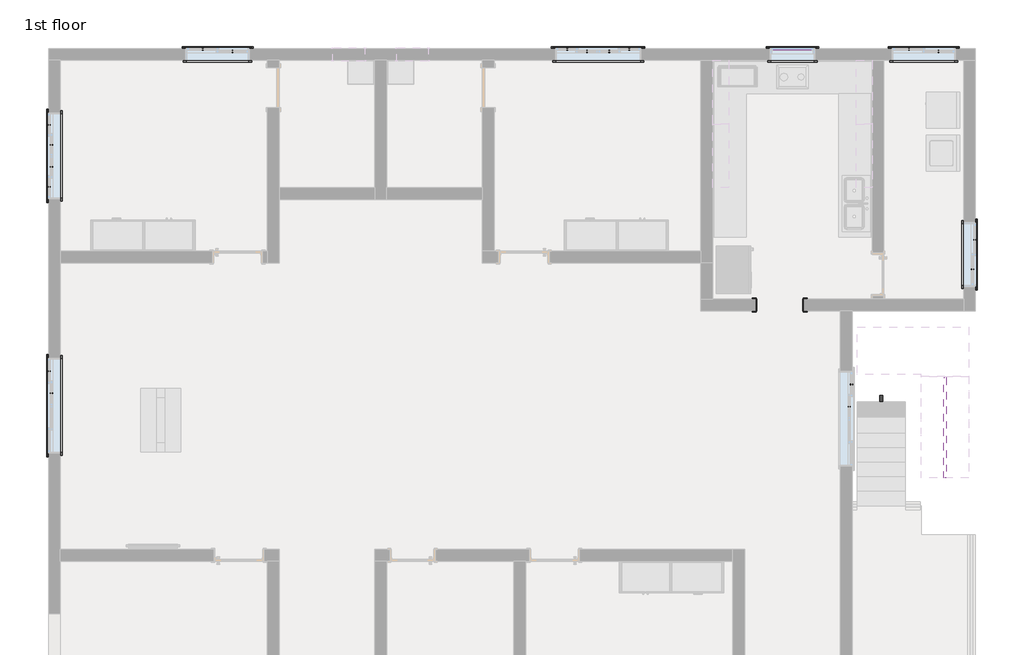
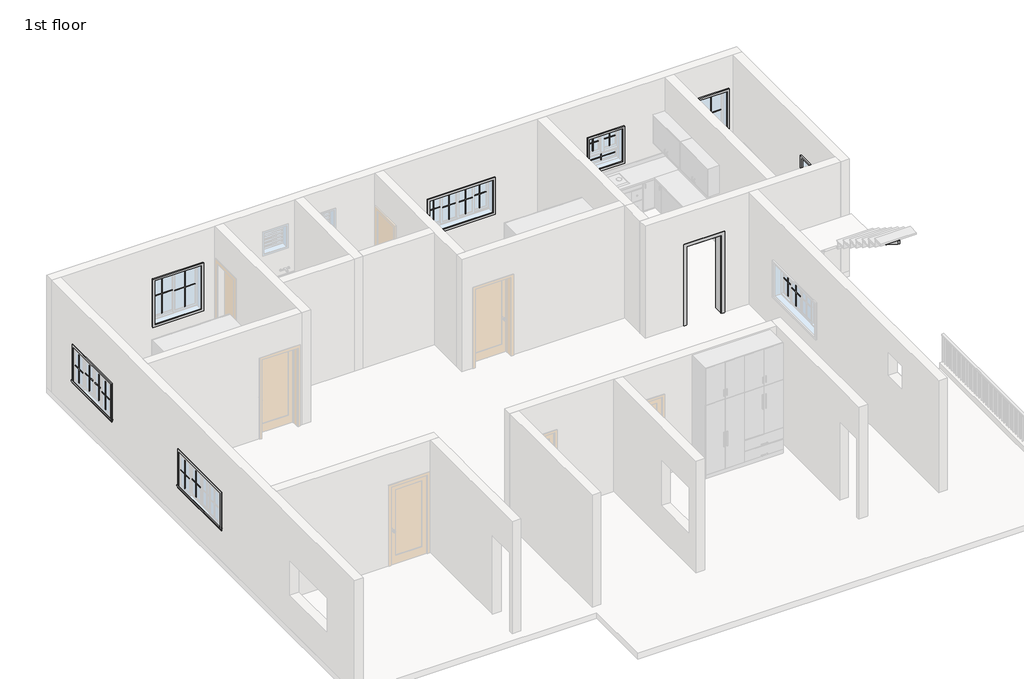
# One storey, part 4 of 4: 36 proxies, 2 members.
"""IFC4 building model written with IfcOpenShell, lengths in millimetres."""

from ifc_helpers import new_model, si_unit, frame, origin, place, context, project, spatial, polyline, outline, extrude, transform, mapped, element, save
from components import muntin_pattern_2x2_muntin_pattern_2x2_6186d23a, muntin_pattern_2x2_muntin_pattern_2x2_31a16349, muntin_pattern_2x2_muntin_pattern_2x2_cf37b409, muntin_pattern_2x2_muntin_pattern_2x2_78ce0566, muntin_pattern_2x2_muntin_pattern_2x2_27bf4e5b, muntin_pattern_2x2_muntin_pattern_2x2_8320156c, proxy_e9bf662a, trim_window_exterior_flat_with_sill_c3f87112, trim_window_exterior_flat_with_sill_3c945769, trim_window_exterior_flat_with_sill_7cfdd449, trim_window_exterior_flat_with_sill_41619996, trim_window_interior_flat_picture_frame_1c33fa8a, trim_window_interior_flat_picture_frame_0edfbaa2, trim_window_interior_flat_picture_frame_f1e0b15b, trim_window_interior_flat_picture_frame_51c85655

model = new_model("IFC4")

# Units and contexts
model_context = context("Model", 3, world=origin())
ifc_project = project(units=[si_unit("LENGTHUNIT", "METRE", prefix="MILLI")], contexts=[model_context])

# Site, building, storey
site = spatial("IfcSite", under=ifc_project)
building = spatial("IfcBuilding", under=site)
storey = spatial("IfcBuildingStorey", under=building, Name="1st floor", Elevation=3810.0)

# Proxies
placement = place(None, origin())
muntin_pattern_2x2_muntin_pattern_2x2_shape = muntin_pattern_2x2_muntin_pattern_2x2_6186d23a(model_context)
element("IfcBuildingElementProxy", 1, Name="Muntin Pattern_2x2 : Muntin Pattern_2x2", ObjectType="Muntin Pattern_2x2 : Muntin Pattern_2x2", at=placement, inside=storey, context=model_context, shape_type="MappedRepresentation", body=[
    mapped(muntin_pattern_2x2_muntin_pattern_2x2_shape, transform((1905.0010838, 7064.4410813, 4806.95), x_axis=(1.0, 0.0, 0.0), y_axis=(0.0, 1.0, 0.0), z_axis=(0.0, 0.0, 1.0))),
])
element("IfcBuildingElementProxy", 2, Name="Muntin Pattern_2x2 : Muntin Pattern_2x2", ObjectType="Muntin Pattern_2x2 : Muntin Pattern_2x2", at=placement, inside=storey, context=model_context, shape_type="MappedRepresentation", body=[
    mapped(muntin_pattern_2x2_muntin_pattern_2x2_shape, transform((2286.0010838, 7019.9910813, 4806.95), x_axis=(1.0, 0.0, 0.0), y_axis=(0.0, 1.0, 0.0), z_axis=(0.0, 0.0, 1.0))),
])
element("IfcBuildingElementProxy", 3, Name="Muntin Pattern_2x2 : Muntin Pattern_2x2", ObjectType="Muntin Pattern_2x2 : Muntin Pattern_2x2", at=placement, inside=storey, context=model_context, shape_type="MappedRepresentation", body=[
    mapped(muntin_pattern_2x2_muntin_pattern_2x2_shape, transform((2711.4510838, 7019.9910813, 4806.95), x_axis=(1.0, 0.0, 0.0), y_axis=(0.0, 1.0, 0.0), z_axis=(0.0, 0.0, 1.0))),
])
element("IfcBuildingElementProxy", 4, Name="Muntin Pattern_2x2 : Muntin Pattern_2x2", ObjectType="Muntin Pattern_2x2 : Muntin Pattern_2x2", at=placement, inside=storey, context=model_context, shape_type="MappedRepresentation", body=[
    mapped(muntin_pattern_2x2_muntin_pattern_2x2_shape, transform((3092.4510838, 7064.4410813, 4806.95), x_axis=(1.0, 0.0, 0.0), y_axis=(0.0, 1.0, 0.0), z_axis=(0.0, 0.0, 1.0))),
])
element("IfcBuildingElementProxy", 5, Name="Muntin Pattern_2x2 : Muntin Pattern_2x2", ObjectType="Muntin Pattern_2x2 : Muntin Pattern_2x2", at=placement, inside=storey, context=model_context, shape_type="MappedRepresentation", body=[
    mapped(muntin_pattern_2x2_muntin_pattern_2x2_shape, transform((-8020.0489162, 4422.8410813, 4806.95), x_axis=(0.0, 1.0, 0.0), y_axis=(-1.0, 0.0, 0.0), z_axis=(0.0, 0.0, 1.0))),
])
element("IfcBuildingElementProxy", 6, Name="Muntin Pattern_2x2 : Muntin Pattern_2x2", ObjectType="Muntin Pattern_2x2 : Muntin Pattern_2x2", at=placement, inside=storey, context=model_context, shape_type="MappedRepresentation", body=[
    mapped(muntin_pattern_2x2_muntin_pattern_2x2_shape, transform((-7975.5989162, 4803.8410813, 4806.95), x_axis=(0.0, 1.0, 0.0), y_axis=(-1.0, 0.0, 0.0), z_axis=(0.0, 0.0, 1.0))),
])
element("IfcBuildingElementProxy", 7, Name="Muntin Pattern_2x2 : Muntin Pattern_2x2", ObjectType="Muntin Pattern_2x2 : Muntin Pattern_2x2", at=placement, inside=storey, context=model_context, shape_type="MappedRepresentation", body=[
    mapped(muntin_pattern_2x2_muntin_pattern_2x2_shape, transform((-7975.5989162, 5229.2910813, 4806.95), x_axis=(0.0, 1.0, 0.0), y_axis=(-1.0, 0.0, 0.0), z_axis=(0.0, 0.0, 1.0))),
])
element("IfcBuildingElementProxy", 8, Name="Muntin Pattern_2x2 : Muntin Pattern_2x2", ObjectType="Muntin Pattern_2x2 : Muntin Pattern_2x2", at=placement, inside=storey, context=model_context, shape_type="MappedRepresentation", body=[
    mapped(muntin_pattern_2x2_muntin_pattern_2x2_shape, transform((-8020.0489162, 5610.2910813, 4806.95), x_axis=(0.0, 1.0, 0.0), y_axis=(-1.0, 0.0, 0.0), z_axis=(0.0, 0.0, 1.0))),
])
muntin_pattern_2x2_muntin_pattern_2x2_2_shape = muntin_pattern_2x2_muntin_pattern_2x2_31a16349(model_context)
element("IfcBuildingElementProxy", 9, Name="Muntin Pattern_2x2 : Muntin Pattern_2x2", ObjectType="Muntin Pattern_2x2 : Muntin Pattern_2x2", at=placement, inside=storey, context=model_context, shape_type="MappedRepresentation", body=[
    mapped(muntin_pattern_2x2_muntin_pattern_2x2_2_shape, transform((-7975.5989162, 463.6160813, 4806.95), x_axis=(0.0, 1.0, 0.0), y_axis=(-1.0, 0.0, 0.0), z_axis=(0.0, 0.0, 1.0))),
])
element("IfcBuildingElementProxy", 10, Name="Muntin Pattern_2x2 : Muntin Pattern_2x2", ObjectType="Muntin Pattern_2x2 : Muntin Pattern_2x2", at=placement, inside=storey, context=model_context, shape_type="MappedRepresentation", body=[
    mapped(muntin_pattern_2x2_muntin_pattern_2x2_2_shape, transform((-8020.0489162, 889.0660813, 4806.95), x_axis=(0.0, 1.0, 0.0), y_axis=(-1.0, 0.0, 0.0), z_axis=(0.0, 0.0, 1.0))),
])
element("IfcBuildingElementProxy", 11, Name="Muntin Pattern_2x2 : Muntin Pattern_2x2", ObjectType="Muntin Pattern_2x2 : Muntin Pattern_2x2", at=placement, inside=storey, context=model_context, shape_type="MappedRepresentation", body=[
    mapped(muntin_pattern_2x2_muntin_pattern_2x2_2_shape, transform((7353.3010838, 635.0660813, 4806.95), x_axis=(0.0, -1.0, 0.0), y_axis=(1.0, 0.0, 0.0), z_axis=(0.0, 0.0, 1.0))),
])
element("IfcBuildingElementProxy", 12, Name="Muntin Pattern_2x2 : Muntin Pattern_2x2", ObjectType="Muntin Pattern_2x2 : Muntin Pattern_2x2", at=placement, inside=storey, context=model_context, shape_type="MappedRepresentation", body=[
    mapped(muntin_pattern_2x2_muntin_pattern_2x2_2_shape, transform((7308.8510838, 209.6160813, 4806.95), x_axis=(0.0, -1.0, 0.0), y_axis=(1.0, 0.0, 0.0), z_axis=(0.0, 0.0, 1.0))),
])
muntin_pattern_2x2_muntin_pattern_2x2_3_shape = muntin_pattern_2x2_muntin_pattern_2x2_cf37b409(model_context)
element("IfcBuildingElementProxy", 13, Name="Muntin Pattern_2x2 : Muntin Pattern_2x2", ObjectType="Muntin Pattern_2x2 : Muntin Pattern_2x2", at=placement, inside=storey, context=model_context, shape_type="MappedRepresentation", body=[
    mapped(muntin_pattern_2x2_muntin_pattern_2x2_3_shape, transform((9018.5885838, 7019.9910813, 4806.95), x_axis=(1.0, 0.0, 0.0), y_axis=(0.0, 1.0, 0.0), z_axis=(0.0, 0.0, 1.0))),
])
element("IfcBuildingElementProxy", 14, Name="Muntin Pattern_2x2 : Muntin Pattern_2x2", ObjectType="Muntin Pattern_2x2 : Muntin Pattern_2x2", at=placement, inside=storey, context=model_context, shape_type="MappedRepresentation", body=[
    mapped(muntin_pattern_2x2_muntin_pattern_2x2_3_shape, transform((8450.2635838, 7064.4410813, 4806.95), x_axis=(1.0, 0.0, 0.0), y_axis=(0.0, 1.0, 0.0), z_axis=(0.0, 0.0, 1.0))),
])
element("IfcBuildingElementProxy", 15, Name="Muntin Pattern_2x2 : Muntin Pattern_2x2", ObjectType="Muntin Pattern_2x2 : Muntin Pattern_2x2", at=placement, inside=storey, context=model_context, shape_type="MappedRepresentation", body=[
    mapped(muntin_pattern_2x2_muntin_pattern_2x2_3_shape, transform((9671.0510838, 2840.1035813, 4806.95), x_axis=(0.0, -1.0, 0.0), y_axis=(1.0, 0.0, 0.0), z_axis=(0.0, 0.0, 1.0))),
])
element("IfcBuildingElementProxy", 16, Name="Muntin Pattern_2x2 : Muntin Pattern_2x2", ObjectType="Muntin Pattern_2x2 : Muntin Pattern_2x2", at=placement, inside=storey, context=model_context, shape_type="MappedRepresentation", body=[
    mapped(muntin_pattern_2x2_muntin_pattern_2x2_3_shape, transform((9715.5010838, 3408.4285813, 4806.95), x_axis=(0.0, -1.0, 0.0), y_axis=(1.0, 0.0, 0.0), z_axis=(0.0, 0.0, 1.0))),
])
element("IfcBuildingElementProxy", 17, Name="Muntin Pattern_2x2 : Muntin Pattern_2x2", ObjectType="Muntin Pattern_2x2 : Muntin Pattern_2x2", at=placement, inside=storey, context=model_context, shape_type="MappedRepresentation", body=[
    mapped(muntin_pattern_2x2_muntin_pattern_2x2_3_shape, transform((-4506.9114162, 7019.9910813, 4806.95), x_axis=(1.0, 0.0, 0.0), y_axis=(0.0, 1.0, 0.0), z_axis=(0.0, 0.0, 1.0))),
])
element("IfcBuildingElementProxy", 18, Name="Muntin Pattern_2x2 : Muntin Pattern_2x2", ObjectType="Muntin Pattern_2x2 : Muntin Pattern_2x2", at=placement, inside=storey, context=model_context, shape_type="MappedRepresentation", body=[
    mapped(muntin_pattern_2x2_muntin_pattern_2x2_3_shape, transform((-5075.2364162, 7064.4410813, 4806.95), x_axis=(1.0, 0.0, 0.0), y_axis=(0.0, 1.0, 0.0), z_axis=(0.0, 0.0, 1.0))),
])
muntin_pattern_2x2_muntin_pattern_2x2_4_shape = muntin_pattern_2x2_muntin_pattern_2x2_78ce0566(model_context)
element("IfcBuildingElementProxy", 19, Name="Muntin Pattern_2x2 : Muntin Pattern_2x2", ObjectType="Muntin Pattern_2x2 : Muntin Pattern_2x2", at=placement, inside=storey, context=model_context, shape_type="MappedRepresentation", body=[
    mapped(muntin_pattern_2x2_muntin_pattern_2x2_4_shape, transform((6005.5135838, 7064.4410813, 5327.65), x_axis=(1.0, 0.0, 0.0), y_axis=(0.0, 1.0, 0.0), z_axis=(0.0, 0.0, 1.0))),
])
muntin_pattern_2x2_muntin_pattern_2x2_5_shape = muntin_pattern_2x2_muntin_pattern_2x2_27bf4e5b(model_context)
element("IfcBuildingElementProxy", 20, Name="Muntin Pattern_2x2 : Muntin Pattern_2x2", ObjectType="Muntin Pattern_2x2 : Muntin Pattern_2x2", at=placement, inside=storey, context=model_context, shape_type="MappedRepresentation", body=[
    mapped(muntin_pattern_2x2_muntin_pattern_2x2_5_shape, transform((6434.1385838, 7064.4410813, 5327.65), x_axis=(-1.0, 0.0, 0.0), y_axis=(0.0, -1.0, 0.0), z_axis=(0.0, 0.0, 1.0))),
])
muntin_pattern_2x2_muntin_pattern_2x2_6_shape = muntin_pattern_2x2_muntin_pattern_2x2_8320156c(model_context)
element("IfcBuildingElementProxy", 21, Name="Muntin Pattern_2x2 : Muntin Pattern_2x2", ObjectType="Muntin Pattern_2x2 : Muntin Pattern_2x2", at=placement, inside=storey, context=model_context, shape_type="MappedRepresentation", body=[
    mapped(muntin_pattern_2x2_muntin_pattern_2x2_6_shape, transform((6219.8260838, 7064.4410813, 5022.85), x_axis=(-1.0, 0.0, 0.0), y_axis=(0.0, -1.0, 0.0), z_axis=(0.0, 0.0, 1.0))),
])
proxy_shape = proxy_e9bf662a(model_context)
element("IfcBuildingElementProxy", 22, Name="Passage Opening-Cased : 36\" x 84\"", ObjectType="Passage Opening-Cased : 36\" x 84\"", at=placement, inside=storey, context=model_context, shape_type="MappedRepresentation", body=[
    mapped(proxy_shape, transform((5970.337427, 2159.0660813, 3810.0), x_axis=(-1.0, 0.0, 0.0), y_axis=(0.0, -1.0, 0.0), z_axis=(0.0, 0.0, 1.0))),
])
trim_window_exterior_flat_with_sill_shape = trim_window_exterior_flat_with_sill_c3f87112(model_context)
element("IfcBuildingElementProxy", 23, Name="Trim-Window-Exterior-Flat : with Sill", ObjectType="Trim-Window-Exterior-Flat : with Sill", at=placement, inside=storey, context=model_context, shape_type="MappedRepresentation", body=[
    mapped(trim_window_exterior_flat_with_sill_shape, transform((2498.7260838, 7073.9660813, 5638.8), x_axis=(-1.0, 0.0, 0.0), y_axis=(0.0, 0.0, 1.0), z_axis=(0.0, 1.0, 0.0))),
])
element("IfcBuildingElementProxy", 24, Name="Trim-Window-Exterior-Flat : with Sill", ObjectType="Trim-Window-Exterior-Flat : with Sill", at=placement, inside=storey, context=model_context, shape_type="MappedRepresentation", body=[
    mapped(trim_window_exterior_flat_with_sill_shape, transform((-8029.5739162, 5016.5660813, 5638.8), x_axis=(0.0, -1.0, 0.0), y_axis=(0.0, 0.0, 1.0), z_axis=(-1.0, 0.0, 0.0))),
])
trim_window_exterior_flat_with_sill_2_shape = trim_window_exterior_flat_with_sill_3c945769(model_context)
element("IfcBuildingElementProxy", 25, Name="Trim-Window-Exterior-Flat : with Sill", ObjectType="Trim-Window-Exterior-Flat : with Sill", at=placement, inside=storey, context=model_context, shape_type="MappedRepresentation", body=[
    mapped(trim_window_exterior_flat_with_sill_2_shape, transform((-8029.5739162, 228.6660813, 5638.8), x_axis=(0.0, -1.0, 0.0), y_axis=(0.0, 0.0, 1.0), z_axis=(-1.0, 0.0, 0.0))),
])
trim_window_exterior_flat_with_sill_3_shape = trim_window_exterior_flat_with_sill_7cfdd449(model_context)
element("IfcBuildingElementProxy", 26, Name="Trim-Window-Exterior-Flat : with Sill", ObjectType="Trim-Window-Exterior-Flat : with Sill", at=placement, inside=storey, context=model_context, shape_type="MappedRepresentation", body=[
    mapped(trim_window_exterior_flat_with_sill_3_shape, transform((8734.4260838, 7073.9660813, 5943.6), x_axis=(-1.0, 0.0, 0.0), y_axis=(0.0, 0.0, 1.0), z_axis=(0.0, 1.0, 0.0))),
])
element("IfcBuildingElementProxy", 27, Name="Trim-Window-Exterior-Flat : with Sill", ObjectType="Trim-Window-Exterior-Flat : with Sill", at=placement, inside=storey, context=model_context, shape_type="MappedRepresentation", body=[
    mapped(trim_window_exterior_flat_with_sill_3_shape, transform((9725.0260838, 3124.2660813, 5943.6), x_axis=(0.0, 1.0, 0.0), y_axis=(0.0, 0.0, 1.0), z_axis=(1.0, 0.0, 0.0))),
])
element("IfcBuildingElementProxy", 28, Name="Trim-Window-Exterior-Flat : with Sill", ObjectType="Trim-Window-Exterior-Flat : with Sill", at=placement, inside=storey, context=model_context, shape_type="MappedRepresentation", body=[
    mapped(trim_window_exterior_flat_with_sill_3_shape, transform((-4791.0739162, 7073.9660813, 5943.6), x_axis=(-1.0, 0.0, 0.0), y_axis=(0.0, 0.0, 1.0), z_axis=(0.0, 1.0, 0.0))),
])
trim_window_exterior_flat_with_sill_4_shape = trim_window_exterior_flat_with_sill_41619996(model_context)
element("IfcBuildingElementProxy", 29, Name="Trim-Window-Exterior-Flat : with Sill", ObjectType="Trim-Window-Exterior-Flat : with Sill", at=placement, inside=storey, context=model_context, shape_type="MappedRepresentation", body=[
    mapped(trim_window_exterior_flat_with_sill_4_shape, transform((6219.8260838, 7073.9660813, 5867.4), x_axis=(-1.0, 0.0, 0.0), y_axis=(0.0, 0.0, 1.0), z_axis=(0.0, 1.0, 0.0))),
])
trim_window_interior_flat_picture_frame_shape = trim_window_interior_flat_picture_frame_1c33fa8a(model_context)
element("IfcBuildingElementProxy", 30, Name="Trim-Window-Interior-Flat : Picture Frame", ObjectType="Trim-Window-Interior-Flat : Picture Frame", at=placement, inside=storey, context=model_context, shape_type="MappedRepresentation", body=[
    mapped(trim_window_interior_flat_picture_frame_shape, transform((2498.7260838, 6845.3660813, 5638.8), x_axis=(1.0, 0.0, 0.0), y_axis=(0.0, 0.0, 1.0), z_axis=(0.0, -1.0, 0.0))),
])
element("IfcBuildingElementProxy", 31, Name="Trim-Window-Interior-Flat : Picture Frame", ObjectType="Trim-Window-Interior-Flat : Picture Frame", at=placement, inside=storey, context=model_context, shape_type="MappedRepresentation", body=[
    mapped(trim_window_interior_flat_picture_frame_shape, transform((-7800.9739162, 5016.5660813, 5638.8), x_axis=(0.0, 1.0, 0.0), y_axis=(0.0, 0.0, 1.0), z_axis=(1.0, 0.0, 0.0))),
])
trim_window_interior_flat_picture_frame_2_shape = trim_window_interior_flat_picture_frame_0edfbaa2(model_context)
element("IfcBuildingElementProxy", 32, Name="Trim-Window-Interior-Flat : Picture Frame", ObjectType="Trim-Window-Interior-Flat : Picture Frame", at=placement, inside=storey, context=model_context, shape_type="MappedRepresentation", body=[
    mapped(trim_window_interior_flat_picture_frame_2_shape, transform((-7800.9739162, 228.6660813, 5638.8), x_axis=(0.0, 1.0, 0.0), y_axis=(0.0, 0.0, 1.0), z_axis=(1.0, 0.0, 0.0))),
])
trim_window_interior_flat_picture_frame_3_shape = trim_window_interior_flat_picture_frame_f1e0b15b(model_context)
element("IfcBuildingElementProxy", 33, Name="Trim-Window-Interior-Flat : Picture Frame", ObjectType="Trim-Window-Interior-Flat : Picture Frame", at=placement, inside=storey, context=model_context, shape_type="MappedRepresentation", body=[
    mapped(trim_window_interior_flat_picture_frame_3_shape, transform((8734.4260838, 6845.3660813, 5943.6), x_axis=(1.0, 0.0, 0.0), y_axis=(0.0, 0.0, 1.0), z_axis=(0.0, -1.0, 0.0))),
])
element("IfcBuildingElementProxy", 34, Name="Trim-Window-Interior-Flat : Picture Frame", ObjectType="Trim-Window-Interior-Flat : Picture Frame", at=placement, inside=storey, context=model_context, shape_type="MappedRepresentation", body=[
    mapped(trim_window_interior_flat_picture_frame_3_shape, transform((9496.4260838, 3124.2660813, 5943.6), x_axis=(0.0, -1.0, 0.0), y_axis=(0.0, 0.0, 1.0), z_axis=(-1.0, 0.0, 0.0))),
])
element("IfcBuildingElementProxy", 35, Name="Trim-Window-Interior-Flat : Picture Frame", ObjectType="Trim-Window-Interior-Flat : Picture Frame", at=placement, inside=storey, context=model_context, shape_type="MappedRepresentation", body=[
    mapped(trim_window_interior_flat_picture_frame_3_shape, transform((-4791.0739162, 6845.3660813, 5943.6), x_axis=(1.0, 0.0, 0.0), y_axis=(0.0, 0.0, 1.0), z_axis=(0.0, -1.0, 0.0))),
])
trim_window_interior_flat_picture_frame_4_shape = trim_window_interior_flat_picture_frame_51c85655(model_context)
element("IfcBuildingElementProxy", 36, Name="Trim-Window-Interior-Flat : Picture Frame", ObjectType="Trim-Window-Interior-Flat : Picture Frame", at=placement, inside=storey, context=model_context, shape_type="MappedRepresentation", body=[
    mapped(trim_window_interior_flat_picture_frame_4_shape, transform((6219.8260838, 6845.3660813, 5867.4), x_axis=(1.0, 0.0, 0.0), y_axis=(0.0, 0.0, 1.0), z_axis=(0.0, -1.0, 0.0))),
])

# Members
element("IfcMember", 37, ObjectType="Carriage - 2\" Width", at=placement, inside=storey, context=model_context, shape_type="SweptSolid", body=[
    extrude(outline(polyline([(825.5660813, 5359.4), (825.5660813, 5263.9282995), (-1459.1783893, 3810.0), (-1657.2839187, 3810.0), (-1657.2839187, 3937.0), (-1377.8839187, 3937.0), (-1377.8839187, 4114.8), (-1098.4839187, 4114.8), (-1098.4839187, 4292.6), (-819.0839187, 4292.6), (-819.0839187, 4470.4), (-539.6839187, 4470.4), (-539.6839187, 4648.2), (-260.2839187, 4648.2), (-260.2839187, 4826.0), (19.1160813, 4826.0), (19.1160813, 5003.8), (298.5160813, 5003.8), (298.5160813, 5181.6), (577.9160813, 5181.6), (577.9160813, 5359.4), (825.5660813, 5359.4)])), frame((7896.2260838, 0.0, 0.0), z_axis=(1.0, 0.0, 0.0), x_axis=(0.0, 1.0, 0.0)), (0.0, 0.0, 1.0), 50.8),
])
element("IfcMember", 38, ObjectType="Carriage - 2\" Width", at=placement, inside=storey, context=model_context, shape_type="SweptSolid", body=[
    extrude(outline(polyline([(-1156.9972984, 6686.3282995), (-1156.9972984, 6781.8), (-909.3472984, 6781.8), (-909.3472984, 6604.0), (-629.9472984, 6604.0), (-629.9472984, 6426.2), (-350.5472984, 6426.2), (-350.5472984, 6248.4), (-71.1472984, 6248.4), (-71.1472984, 6070.6), (208.2527016, 6070.6), (208.2527016, 5892.8), (487.6527016, 5892.8), (487.6527016, 5715.0), (767.0527016, 5715.0), (767.0527016, 5461.932845), (-1156.9972984, 6686.3282995)])), frame((9115.4260838, 0.0, 0.0), z_axis=(1.0, 0.0, 0.0), x_axis=(0.0, 1.0, 0.0)), (0.0, 0.0, 1.0), 50.8),
])

save(model, "model.ifc")

# Revit data of these elements
# Type "Muntin Pattern_2x2 : Muntin Pattern_2x2"
#   Width [instance default] = 4' - 0"
#   Thickness = 0' - 0 1/2"
#   Height [instance default] = 4' - 0"
#   Distance = 0' - 0 3/4"
#   Interior Material [instance default] = none
#   Exterior Material [instance default] = none
#   Default Elevation = 0
# Type "Passage Opening-Cased : 36\" x 84\""
#   Height = 7' - 0"
#   Trim Thickness = 0' - 0 3/4"
#   Trim Width = 0' - 3"
#   Width = 3' - 0"
#   Frame Material = Door - Frame
#   Default Elevation = 0
# Type "Trim-Window-Exterior-Flat : with Sill"
#   Trim Width = 0' - 2 1/4"
#   Trim Thickness_Picture Frame = 0' - 1 1/4"
#   Trim Thickness_with Sill = 0' - 0 3/4"
#   Sill Thickness = 0' - 1 1/4"
#   Opening Width [instance default] = 2' - 0"
#   Opening Height [instance default] = 3' - 0"
#   Default Elevation = 4' - 0"
#   Sill = yes
#   Picture Frame = no
#   Trim Material [instance default] = none
# Type "Trim-Window-Interior-Flat : Picture Frame"
#   Trim Thickness_Picture Frame = 0' - 1 1/4"
#   Trim Width = 0' - 2 1/4"
#   Trim Thickness_with Sill = 0' - 0 3/4"
#   Sill Thickness = 0' - 1 1/4"
#   Opening Width [instance default] = 2' - 0"
#   Opening Height [instance default] = 3' - 0"
#   Default Elevation = 4' - 0"
#   Sill = no
#   Picture Frame = yes
#   Trim Material [instance default] = none
# Elements 1, 2, 3, 4, 5, 6, 7, 8 (IfcBuildingElementProxy, "Muntin Pattern_2x2 : Muntin Pattern_2x2")
#   Width = 1' - 1 1/4"
#   Height = 2' - 6 1/4"
#   Interior Material = Wood - Stained
#   Exterior Material = Clad - White
#   Phase Created = New Construction
#   Materials on its faces: "Clad - White", "Wood - Stained"
# Elements 9, 10, 11, 12 (IfcBuildingElementProxy, "Muntin Pattern_2x2 : Muntin Pattern_2x2")
#   Width = 1' - 3"
#   Height = 2' - 6 1/4"
#   Interior Material = Wood - Stained
#   Exterior Material = Clad - White
#   Phase Created = New Construction
#   Materials on its faces: "Clad - White", "Wood - Stained"
# Elements 13, 14, 15, 16, 17, 18 (IfcBuildingElementProxy, "Muntin Pattern_2x2 : Muntin Pattern_2x2")
#   Width = 1' - 8 5/8"
#   Height = 3' - 6 1/4"
#   Interior Material = Wood - Stained
#   Exterior Material = Clad - White
#   Phase Created = New Construction
#   Materials on its faces: "Clad - White", "Wood - Stained"
# Elements 19, 20 (IfcBuildingElementProxy, "Muntin Pattern_2x2 : Muntin Pattern_2x2")
#   Width = 0' - 11 5/8"
#   Height = 1' - 6 1/2"
#   Interior Material = Wood - Stained
#   Exterior Material = Clad - White
#   Phase Created = New Construction
#   Materials on its faces: "Clad - White", "Wood - Stained"
# Element 21 (IfcBuildingElementProxy, "Muntin Pattern_2x2 : Muntin Pattern_2x2")
#   Width = 2' - 4 1/2"
#   Height = 0' - 6 1/2"
#   Interior Material = Wood - Stained
#   Exterior Material = Clad - White
#   Phase Created = New Construction
#   Materials on its faces: "Clad - White", "Wood - Stained"
# Element 22 (IfcBuildingElementProxy, "Passage Opening-Cased : 36\" x 84\"")
#   Phase Created = New Construction
#   Materials on its faces: "Door - Frame"
# Elements 23, 24 (IfcBuildingElementProxy, "Trim-Window-Exterior-Flat : with Sill")
#   Opening Width = 5' - 5"
#   Opening Height = 3' - 0"
#   Trim Material = Clad - White
#   Phase Created = New Construction
#   Materials on its faces: "Clad - White"
# Element 25 (IfcBuildingElementProxy, "Trim-Window-Exterior-Flat : with Sill")
#   Opening Width = 6' - 0"
#   Opening Height = 3' - 0"
#   Trim Material = Clad - White
#   Phase Created = New Construction
#   Materials on its faces: "Clad - White"
# Elements 26, 27, 28 (IfcBuildingElementProxy, "Trim-Window-Exterior-Flat : with Sill")
#   Opening Width = 4' - 0"
#   Opening Height = 4' - 0"
#   Trim Material = Clad - White
#   Phase Created = New Construction
#   Materials on its faces: "Clad - White"
# Element 29 (IfcBuildingElementProxy, "Trim-Window-Exterior-Flat : with Sill")
#   Opening Width = 2' - 10"
#   Opening Height = 3' - 0"
#   Trim Material = Clad - White
#   Phase Created = New Construction
#   Materials on its faces: "Clad - White"
# Elements 30, 31 (IfcBuildingElementProxy, "Trim-Window-Interior-Flat : Picture Frame")
#   Opening Width = 5' - 5"
#   Opening Height = 3' - 0"
#   Trim Material = Wood - Stained
#   Phase Created = New Construction
#   Materials on its faces: "Wood - Stained"
# Element 32 (IfcBuildingElementProxy, "Trim-Window-Interior-Flat : Picture Frame")
#   Opening Width = 6' - 0"
#   Opening Height = 3' - 0"
#   Trim Material = Wood - Stained
#   Phase Created = New Construction
#   Materials on its faces: "Wood - Stained"
# Elements 33, 34, 35 (IfcBuildingElementProxy, "Trim-Window-Interior-Flat : Picture Frame")
#   Opening Width = 4' - 0"
#   Opening Height = 4' - 0"
#   Trim Material = Wood - Stained
#   Phase Created = New Construction
#   Materials on its faces: "Wood - Stained"
# Element 36 (IfcBuildingElementProxy, "Trim-Window-Interior-Flat : Picture Frame")
#   Opening Width = 2' - 10"
#   Opening Height = 3' - 0"
#   Trim Material = Wood - Stained
#   Phase Created = New Construction
#   Materials on its faces: "Wood - Stained"
# Elements 37, 38 (IfcMember, "Carriage - 2\" Width")
#   Phase Created = New Construction
# Materials
#   "Door - Frame": colour RGB 118 70 51, transparency 0, Cost = 0
#   "Clad - White": class "Wood", colour RGB 242 242 238, transparency 0, Cost = 0
#   "Wood - Stained": class "Wood", colour RGB 224 178 126, transparency 0, Cost = 0
